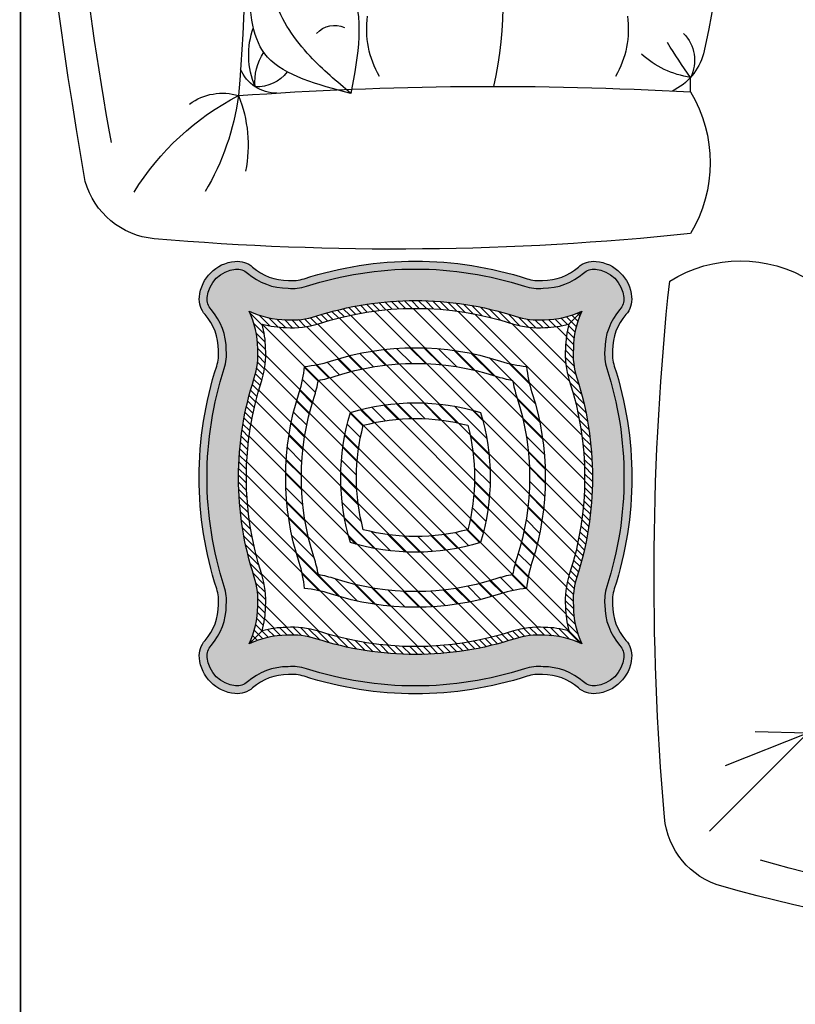
# Model space of a CAD drawing. Units: inches. Extents: x 844 to 2234, y 346 to 1084.
# Tile 50 of 93: x 1843 to 1859, y 668 to 688. Entities that reach past the tile are written whole.
import ezdxf

# ---------------------------------------------------------------- set-up
doc = ezdxf.new("R2010")
doc.units = ezdxf.units.IN
doc.header["$MEASUREMENT"] = 0
doc.layers.add('A-WALL', color=7, linetype='Continuous', lineweight=35)
doc.layers.add('furniture', color=8, linetype='Continuous', lineweight=18)
for name, color, linetype in [('RA-AP-01$0$FURN', 3, 'Continuous'), ('RA-AP-01$0$steel', 193, 'Continuous'), ('RA-AP-01$0$WOOD', 64, 'Continuous')]:
    doc.layers.add(name, color=color, linetype=linetype)
pattern_1 = [(45, (0, 1.362436106329781), (-0.0088388347648318, 0.0088388347648318), [])]
pattern_2 = [(45, (0, 1.362436106329781), (-0.0044194173824159, 0.0044194173824159), [])]

# ---------------------------------------------------------------- blocks, each defined once
blk = doc.blocks.new('A$C2FCF5309')
at = {"layer": 'RA-AP-01$0$FURN'}
h = blk.add_hatch(dxfattribs=at)
h.set_pattern_fill('ANSI31', color=256, scale=0.1, style=0)
h.set_pattern_definition(pattern_1)
h.paths.add_polyline_path([(5.038683893313746, -5.169250834004607, -0.1583983521602212), (5.038683893312098, -5.373464580902012, 0.0306258898943267), (5.033304057242972, -5.394827569605182, 0.0306258898948892), (5.01194106853941, -5.40020740567441, -0.1028142994996694), (4.878286182323899, -5.414871334512708), (4.863600873530158, -5.43331743520547, 0.1120482678681049), (5.018059823131753, -5.419248541734471, -0.052642197802937), (5.050972078299936, -5.412495590662115, -0.0526421977994963), (5.057725029371615, -5.379583335496025, 0.1583028414702701), (5.057725029372958, -5.163132079409654, -0.052642197806903), (5.050972078299777, -5.130219824239078, -0.0526421977995126), (5.018059823133679, -5.123466873167369, 0.0215995840215353), (4.988903013548211, -5.115372132362452), (4.975007495303644, -5.132826183367946, -0.0289147572844802), (5.011941068537408, -5.142508009226167, 0.0306258898976746), (5.033304057242868, -5.147887845296027, 0.0306258899022411)])
h.paths.add_polyline_path([(4.975007495303645, -5.132826183367946), (4.988903013548211, -5.115372132362452, 0.1362374241599938), (4.801608567045604, -5.12346687316654, -0.0526421978036853), (4.768696311876971, -5.130219824239102, -0.05264219780204), (4.761943360804856, -5.163132079406747, 0.1583028414743723), (4.761943360806116, -5.379583335498449, -0.0526421977955461), (4.768696311877141, -5.412495590662114, -0.0526421978073986), (4.801608567048022, -5.419248541735437, 0.0454484293938888), (4.863600873530158, -5.43331743520547), (4.878286182323899, -5.414871334512708, -0.0546933379798044), (4.80772732164382, -5.40020740567649, 0.030625889903973), (4.786364332934043, -5.394827569605216, 0.0306258898932853), (4.780984496865101, -5.373464580902791, -0.1583983521638281), (4.780984496864308, -5.169250834000963, 0.03062588989692), (4.786364332933943, -5.147887845296004, 0.0306258898946324), (4.807727321637318, -5.142508009226805, -0.1288932573266927)])
h.paths.add_polyline_path([(4.843422214712861, -5.204945727074827, -0.0783685831716868), (4.924134454130224, -5.196727409635105), (4.939146578618322, -5.177870798323143, 0.1012675676854134), (4.827248748758957, -5.188772261120899, 0.1253648873081696), (4.820394258584192, -5.327034652050361), (4.837127701354095, -5.306015906404253, -0.0981593964869636)], flags=17)
h.paths.add_polyline_path([(4.843422214712824, -5.337769687826355, -0.0311091841722656), (4.837127701354095, -5.306015906404253), (4.820394258584193, -5.32703465205036, 0.0247727657431944), (4.827248748758908, -5.353943153780261, 0.0812754385032542), (4.916962478476905, -5.36629034358622), (4.933684093813825, -5.345286454285511, -0.0876255421014372)], flags=17)
h.paths.add_polyline_path([(4.992419641418037, -5.353943153780226, 0.1506053783834298), (4.992419641417933, -5.188772261120954, 0.0485966419124224), (4.939146578618321, -5.177870798323143), (4.924134454130224, -5.196727409635105, -0.0507799419579301), (4.976246175464031, -5.204945727074882, -0.1296645318906876), (4.97624617546411, -5.337769687826316, -0.0415667119298777), (4.933684093813825, -5.345286454285511), (4.916962478476905, -5.36629034358622, 0.0684915676023693)], flags=17)
h = blk.add_hatch(dxfattribs=at)
h.set_pattern_fill('ANSI31', color=256, scale=0.1, style=0)
h.set_pattern_definition(pattern_1)
h.paths.add_polyline_path([(5.038683893313746, -5.169250834004607, -0.1583983521602212), (5.038683893312098, -5.373464580902012, 0.0306258898943267), (5.033304057242972, -5.394827569605182, 0.0306258898948892), (5.01194106853941, -5.40020740567441, -0.1028142994996694), (4.878286182323899, -5.414871334512708), (4.863600873530158, -5.43331743520547, 0.1120482678681049), (5.018059823131753, -5.419248541734471, -0.052642197802937), (5.050972078299936, -5.412495590662115, -0.0526421977994963), (5.057725029371615, -5.379583335496025, 0.1583028414702701), (5.057725029372958, -5.163132079409654, -0.052642197806903), (5.050972078299777, -5.130219824239078, -0.0526421977995126), (5.018059823133679, -5.123466873167369, 0.0215995840215353), (4.988903013548211, -5.115372132362452), (4.975007495303644, -5.132826183367946, -0.0289147572844802), (5.011941068537408, -5.142508009226167, 0.0306258898976746), (5.033304057242868, -5.147887845296027, 0.0306258899022411)])
h.paths.add_polyline_path([(4.975007495303645, -5.132826183367946), (4.988903013548211, -5.115372132362452, 0.1362374241599938), (4.801608567045604, -5.12346687316654, -0.0526421978036853), (4.768696311876971, -5.130219824239102, -0.05264219780204), (4.761943360804856, -5.163132079406747, 0.1583028414743723), (4.761943360806116, -5.379583335498449, -0.0526421977955461), (4.768696311877141, -5.412495590662114, -0.0526421978073986), (4.801608567048022, -5.419248541735437, 0.0454484293938888), (4.863600873530158, -5.43331743520547), (4.878286182323899, -5.414871334512708, -0.0546933379798044), (4.80772732164382, -5.40020740567649, 0.030625889903973), (4.786364332934043, -5.394827569605216, 0.0306258898932853), (4.780984496865101, -5.373464580902791, -0.1583983521638281), (4.780984496864308, -5.169250834000963, 0.03062588989692), (4.786364332933943, -5.147887845296004, 0.0306258898946324), (4.807727321637318, -5.142508009226805, -0.1288932573266927)])
h.paths.add_polyline_path([(4.843422214712861, -5.204945727074827, -0.0783685831716868), (4.924134454130224, -5.196727409635105), (4.939146578618322, -5.177870798323143, 0.1012675676854134), (4.827248748758957, -5.188772261120899, 0.1253648873081696), (4.820394258584192, -5.327034652050361), (4.837127701354095, -5.306015906404253, -0.0981593964869636)], flags=17)
h.paths.add_polyline_path([(4.843422214712824, -5.337769687826355, -0.0311091841722656), (4.837127701354095, -5.306015906404253), (4.820394258584193, -5.32703465205036, 0.0247727657431944), (4.827248748758908, -5.353943153780261, 0.0812754385032542), (4.916962478476905, -5.36629034358622), (4.933684093813825, -5.345286454285511, -0.0876255421014372)], flags=17)
h.paths.add_polyline_path([(4.992419641418037, -5.353943153780226, 0.1506053783834298), (4.992419641417933, -5.188772261120954, 0.0485966419124224), (4.939146578618321, -5.177870798323143), (4.924134454130224, -5.196727409635105, -0.0507799419579301), (4.976246175464031, -5.204945727074882, -0.1296645318906876), (4.97624617546411, -5.337769687826316, -0.0415667119298777), (4.933684093813825, -5.345286454285511), (4.916962478476905, -5.36629034358622, 0.0684915676023693)], flags=17)
at = {"layer": 'RA-AP-01$0$WOOD'}
h = blk.add_hatch(color=256, dxfattribs=at)
edge = h.paths.add_edge_path()
edge.add_arc((4.683001772622394, -5.026441828662609), 0.0299999999999998, 48.77105092035535, 95.25687599427813)
edge.add_arc((4.684834195088484, -5.046357707450686), 0.0499999999998897, 95.25687599443106, 174.7431240064049)
edge.add_arc((4.664918316300367, -5.044525284985046), 0.0300000000000005, 174.7431240062535, 221.2289490796905)
edge.add_arc((4.591236830209155, -5.109094338216345), 0.0679700159630267, -0.5333070513215148, 41.228949079691915, ccw=False)
edge.add_arc((4.609451302807284, -5.114694777173187), 0.0500000000000008, -17.3556839752095, 5.7020707654044145, ccw=False)
edge.add_arc((5.095208119646659, -5.271357707450659), 0.4603971832811796, 162.0683908477609, 197.9316091523306)
edge.add_arc((4.609451302807533, -5.428020637728902), 0.0500000000000006, -5.702070765320514, 17.355683975293914, ccw=False)
edge.add_arc((4.591236830209412, -5.433621076685779), 0.0679700159630261, -41.228949079600625, 0.5333070514128053, ccw=False)
edge.add_arc((4.664918316300727, -5.498190129916959), 0.0299999999999995, 138.7710509204022, 185.256875994324)
edge.add_arc((4.684834195088642, -5.496357707450695), 0.0499999999997451, 185.2568759946742, 264.74312400432)
edge.add_arc((4.683001772622394, -5.516273586238612), 0.03, 264.743124003969, 311.2289490796446)
edge.add_arc((4.747570825853633, -5.589955072329876), 0.0679700159630271, 89.4666929486321, 131.2289490796457, ccw=False)
edge.add_arc((4.753171264810493, -5.57174059973175), 0.0500000000000015, 72.64431602474701, 95.70207076536133, ccw=False)
edge.add_arc((4.909834195088355, -5.085983782892503), 0.4603971832811774, 252.0683908477147, 287.9316091522845)
edge.add_arc((5.06649712536621, -5.57174059973175), 0.0499999999999999, 84.29792923463953, 107.35568397525361, ccw=False)
edge.add_arc((5.072097564323069, -5.589955072329877), 0.0679700159630274, 48.771050920354185, 90.5333070513679, ccw=False)
edge.add_arc((5.136666617554309, -5.516273586238614), 0.0299999999999997, 228.771050920353, 275.2568759942969)
edge.add_arc((5.134834195088338, -5.496357707450417), 0.0499999999999982, 275.2568759942949, 354.7431240057633)
edge.add_arc((5.154750073876535, -5.498190129916372), 0.0299999999999999, 354.7431240057662, 401.2289490796891)
edge.add_arc((5.228431559967749, -5.433621076685074), 0.0679700159630274, 179.4666929486771, 221.2289490796903, ccw=False)
edge.add_arc((5.210217087369615, -5.428020637728227), 0.0499999999999976, 162.6443160247947, 185.7020707654089, ccw=False)
edge.add_arc((4.724460270530244, -5.271357707450757), 0.4603971832811793, 342.0683908477607, 377.9316091523305)
edge.add_arc((5.210217087369368, -5.114694777172509), 0.0500000000000019, 174.2979292346878, 197.355683975302, ccw=False)
edge.add_arc((5.228431559967489, -5.109094338215639), 0.0679700159630279, 138.7710509203993, 180.5333070514128, ccw=False)
edge.add_arc((5.154750073876174, -5.044525284984457), 0.0300000000000001, 318.771050920401, 365.2568759954636)
edge.add_arc((5.13483419508816, -5.046357707450624), 0.0499999999998349, 5.256875995237118, 84.74312400549572)
edge.add_arc((5.136666617554308, -5.026441828662608), 0.0299999999999994, 84.74312400572185, 131.2289490796446)
edge.add_arc((5.072097564323072, -4.952760342571343), 0.0679700159630261, 269.4666929486298, 311.22894907964354, ccw=False)
edge.add_arc((5.066497125366206, -4.97097481516947), 0.0499999999999992, 252.64431602475162, 275.70207076536565, ccw=False)
edge.add_arc((4.909834195088355, -5.456731632008717), 0.4603971832811764, 72.06839084771546, 107.9316091522853)
edge.add_arc((4.753171264810493, -4.970974815169471), 0.0500000000000016, 264.2979292346387, 287.355683975253, ccw=False)
edge.add_arc((4.747570825853633, -4.952760342571346), 0.0679700159630274, 228.7710509203543, 270.5333070513679, ccw=False)
edge = h.paths.add_edge_path(flags=16)
edge.add_arc((4.683001772622395, -5.026441828662608), 0.019999999999999, 48.7710509203555, 95.2568759942793)
edge.add_arc((4.684834195088469, -5.046357707450671), 0.0399999999998731, 95.2568759944489, 174.7431240064248)
edge.add_arc((4.664918316300404, -5.044525284985035), 0.020000000000036, 174.7431240062186, 221.2289490796461)
edge.add_arc((4.591236830209151, -5.109094338216346), 0.0779700159630296, -0.13764630038667747, 41.228949079689585, ccw=False)
edge.add_arc((4.609451302807307, -5.11469477717304), 0.060000000000024, -17.406127045137907, 5.176192161068002, ccw=False)
edge.add_arc((5.09520811964665, -5.271357707450659), 0.4503971832811708, 162.0623235129628, 197.9376764869162)
edge.add_arc((4.609451302807532, -5.428020637728943), 0.0599999999999982, -5.176192160466428, 17.406127046715312, ccw=False)
edge.add_arc((4.591236830209414, -5.433621076685778), 0.0779700159630257, -41.2289490796029, 0.13764630095249686, ccw=False)
edge.add_arc((4.664918316300731, -5.498190129916961), 0.0200000000000047, 138.7710509204103, 185.2568759943212)
edge.add_arc((4.684834195088606, -5.496357707450731), 0.0399999999997066, 185.2568759947174, 264.7431240043665)
edge.add_arc((4.683001772622369, -5.516273586238541), 0.020000000000069, 264.7431240038842, 311.2289490795622)
edge.add_arc((4.747570825853635, -5.589955072329884), 0.0779700159630344, 89.8623536987642, 131.2289490796432, ccw=False)
edge.add_arc((4.753171264810603, -5.571740599731771), 0.0599999999999895, 72.5938729544394, 95.1761921602253, ccw=False)
edge.add_arc((4.909834195088365, -5.085983782892505), 0.4503971832811724, 252.0623235129989, 287.9376764870498)
edge.add_arc((5.066497125366216, -5.571740599731755), 0.0600000000000047, 84.8238078399923, 107.40612704528041, ccw=False)
edge.add_arc((5.072097564322998, -5.589955072329853), 0.077970015963056, 48.771050920303594, 90.13764630126451, ccw=False)
edge.add_arc((5.136666617554307, -5.516273586238622), 0.0199999999999931, 228.771050920344, 275.2568759943037)
edge.add_arc((5.134834195088338, -5.496357707450416), 0.0400000000000004, 275.2568759942928, 354.7431240057607)
edge.add_arc((5.154750073876533, -5.498190129916375), 0.0200000000000037, 354.7431240057783, 401.2289490796939)
edge.add_arc((5.228431559967745, -5.433621076685076), 0.0779700159630239, 179.8623536995147, 221.2289490796908, ccw=False)
edge.add_arc((5.210217087369586, -5.428020637728345), 0.0600000000000054, 162.5938729554486, 185.1761921609759, ccw=False)
edge.add_arc((4.724460270530243, -5.271357707450766), 0.4503971832811826, 342.0623235128896, 377.937676486982)
edge.add_arc((5.210217087369347, -5.114694777172486), 0.0599999999999777, 174.8238078387611, 197.4061270462219, ccw=False)
edge.add_arc((5.228431559967523, -5.109094338215542), 0.0779700159629885, 138.7710509204687, 180.1376463004423, ccw=False)
edge.add_arc((5.154750073876175, -5.044525284984459), 0.0199999999999989, 318.771050920406, 365.2568759954698)
edge.add_arc((5.134834195088138, -5.046357707450646), 0.0399999999998586, 5.256875995208452, 84.74312400546732)
edge.add_arc((5.136666617554292, -5.02644182866256), 0.0199999999999529, 84.74312400577769, 131.2289490797025)
edge.add_arc((5.072097564323069, -4.952760342571338), 0.077970015963032, 269.86235369901414, 311.2289490796421, ccw=False)
edge.add_arc((5.06649712536618, -4.97097481516946), 0.0600000000000007, 252.5938729548277, 275.17619216047467, ccw=False)
edge.add_arc((4.909834195088353, -5.456731632008716), 0.4503971832811739, 72.06232351293887, 107.9376764867365)
edge.add_arc((4.753171264810429, -4.970974815169467), 0.0599999999999991, 264.82380783985815, 287.40612704769893, ccw=False)
edge.add_arc((4.747570825853681, -4.952760342571361), 0.0779700159630467, 228.7710509203206, 270.13764630113724, ccw=False)
h = blk.add_hatch(color=256, dxfattribs=at)
edge = h.paths.add_edge_path()
edge.add_arc((4.683001772622395, -5.026441828662608), 0.019999999999999, 48.7710509203555, 95.2568759942793)
edge.add_arc((4.684834195088469, -5.046357707450671), 0.0399999999998731, 95.2568759944489, 174.7431240064248)
edge.add_arc((4.664918316300404, -5.044525284985035), 0.020000000000036, 174.7431240062186, 221.2289490796461)
edge.add_arc((4.591236830209151, -5.109094338216346), 0.0779700159630296, -0.13764630038667747, 41.228949079689585, ccw=False)
edge.add_arc((4.609451302807307, -5.11469477717304), 0.060000000000024, -17.406127045137907, 5.176192161068002, ccw=False)
edge.add_arc((5.09520811964665, -5.271357707450659), 0.4503971832811708, 162.0623235129628, 197.9376764869162)
edge.add_arc((4.609451302807532, -5.428020637728943), 0.0599999999999982, -5.176192160466428, 17.406127046715312, ccw=False)
edge.add_arc((4.591236830209414, -5.433621076685778), 0.0779700159630257, -41.2289490796029, 0.13764630095249686, ccw=False)
edge.add_arc((4.664918316300731, -5.498190129916961), 0.0200000000000047, 138.7710509204103, 185.2568759943212)
edge.add_arc((4.684834195088606, -5.496357707450731), 0.0399999999997066, 185.2568759947174, 264.7431240043665)
edge.add_arc((4.683001772622369, -5.516273586238541), 0.020000000000069, 264.7431240038842, 311.2289490795622)
edge.add_arc((4.747570825853635, -5.589955072329884), 0.0779700159630344, 89.8623536987642, 131.2289490796432, ccw=False)
edge.add_arc((4.753171264810603, -5.571740599731771), 0.0599999999999895, 72.5938729544394, 95.1761921602253, ccw=False)
edge.add_arc((4.909834195088365, -5.085983782892505), 0.4503971832811724, 252.0623235129989, 287.9376764870498)
edge.add_arc((5.066497125366216, -5.571740599731755), 0.0600000000000047, 84.8238078399923, 107.40612704528041, ccw=False)
edge.add_arc((5.072097564322998, -5.589955072329853), 0.077970015963056, 48.771050920303594, 90.13764630126451, ccw=False)
edge.add_arc((5.136666617554307, -5.516273586238622), 0.0199999999999931, 228.771050920344, 275.2568759943037)
edge.add_arc((5.134834195088338, -5.496357707450416), 0.0400000000000004, 275.2568759942928, 354.7431240057607)
edge.add_arc((5.154750073876533, -5.498190129916375), 0.0200000000000037, 354.7431240057783, 401.2289490796939)
edge.add_arc((5.228431559967745, -5.433621076685076), 0.0779700159630239, 179.8623536995147, 221.2289490796908, ccw=False)
edge.add_arc((5.210217087369586, -5.428020637728345), 0.0600000000000054, 162.5938729554486, 185.1761921609759, ccw=False)
edge.add_arc((4.724460270530243, -5.271357707450766), 0.4503971832811826, 342.0623235128896, 377.937676486982)
edge.add_arc((5.210217087369347, -5.114694777172486), 0.0599999999999777, 174.8238078387611, 197.4061270462219, ccw=False)
edge.add_arc((5.228431559967523, -5.109094338215542), 0.0779700159629885, 138.7710509204687, 180.1376463004423, ccw=False)
edge.add_arc((5.154750073876175, -5.044525284984459), 0.0199999999999989, 318.771050920406, 365.2568759954698)
edge.add_arc((5.134834195088138, -5.046357707450646), 0.0399999999998586, 5.256875995208452, 84.74312400546732)
edge.add_arc((5.136666617554292, -5.02644182866256), 0.0199999999999529, 84.74312400577769, 131.2289490797025)
edge.add_arc((5.072097564323069, -4.952760342571338), 0.077970015963032, 269.86235369901414, 311.2289490796421, ccw=False)
edge.add_arc((5.06649712536618, -4.97097481516946), 0.0600000000000007, 252.5938729548277, 275.17619216047467, ccw=False)
edge.add_arc((4.909834195088353, -5.456731632008716), 0.4503971832811739, 72.06232351293887, 107.9376764867365)
edge.add_arc((4.753171264810429, -4.970974815169467), 0.0599999999999991, 264.82380783985815, 287.40612704769893, ccw=False)
edge.add_arc((4.747570825853681, -4.952760342571361), 0.0779700159630467, 228.7710509203206, 270.13764630113724, ccw=False)
edge = h.paths.add_edge_path(flags=16)
edge.add_arc((4.591236830209151, -5.109094338216348), 0.1179700159630308, 0.7417751874182841, 24.563326950263672, ccw=False)
edge.add_arc((4.609451302807302, -5.114694777173093), 0.100000000000012, -17.52836504564658, 4.087328884225087, ccw=False)
edge.add_arc((5.095208119646651, -5.271357707450657), 0.4103971832811724, 162.0403002448777, 197.9596997550675)
edge.add_arc((4.60945130280753, -5.428020637728918), 0.1000000000000027, -4.087328883827581, 17.528365046291924, ccw=False)
edge.add_arc((4.591236830209414, -5.433621076685779), 0.1179700159630246, 335.43667305041845, 359.2582248129738, ccw=False)
edge.add_arc((4.747570825853596, -5.589955072329891), 0.117970015963042, 90.7417751868461, 114.5633269496104, ccw=False)
edge.add_arc((4.753171264810559, -5.571740599731767), 0.0999999999999976, 72.47163495370341, 94.0873288836737, ccw=False)
edge.add_arc((4.909834195088367, -5.085983782892503), 0.4103971832811735, 252.0403002449999, 287.9596997551833)
edge.add_arc((5.066497125366205, -5.571740599731755), 0.1000000000000057, 85.91267111645209, 107.5283650455624, ccw=False)
edge.add_arc((5.072097564322985, -5.58995507232986), 0.117970015963046, 65.4366730497672, 89.25822481317113, ccw=False)
edge.add_arc((5.22843155996773, -5.433621076684992), 0.1179700159630096, 180.7417751873964, 204.5633269502712, ccw=False)
edge.add_arc((5.210217087369591, -5.428020637728301), 0.0999999999999969, 162.4716349546276, 184.0873288841682, ccw=False)
edge.add_arc((4.724460270530243, -5.271357707450766), 0.4103971832811825, 342.0403002448147, 377.9596997550345)
edge.add_arc((5.210217087369347, -5.114694777172489), 0.0999999999999796, 175.9126711156995, 197.5283650464392, ccw=False)
edge.add_arc((5.228431559967512, -5.109094338215525), 0.1179700159630019, 155.4366730502992, 179.2582248126247, ccw=False)
edge.add_arc((5.072097564323172, -4.952760342571314), 0.1179700159630537, 270.74177518697286, 294.56332694975765, ccw=False)
edge.add_arc((5.066497125366189, -4.970974815169462), 0.1000000000000017, 252.471634954247, 274.0873288838353, ccw=False)
edge.add_arc((4.909834195088353, -5.456731632008716), 0.4103971832811758, 72.04030024486342, 107.9596997549354)
edge.add_arc((4.75317126481046, -4.970974815169467), 0.1000000000000041, 265.91267111635307, 287.5283650466103, ccw=False)
edge.add_arc((4.747570825853629, -4.952760342571342), 0.1179700159630538, 245.43667304992562, 269.2582248131125, ccw=False)
h = blk.add_hatch(dxfattribs=at)
h.set_pattern_fill('ANSI31', color=256, scale=0.05, style=0)
h.set_pattern_definition(pattern_2)
h.paths.add_polyline_path([(5.105336294329346, -5.394854099602528, 0.0940138826956367), (5.100476366643778, -5.435568764288975, 0.0606271852326483), (5.104678567100611, -5.466202079462671, 0.0606271852344644), (5.074045251925975, -5.46199987900586, 0.0940138827021426), (5.033330587236848, -5.466859806692645, -0.1305325492494615), (4.828072633169377, -5.477944178050054), (4.821119726105699, -5.486677669841435, 0.1336226599878005), (5.036379334063467, -5.476383803188216, -0.0945969211935747), (5.073624810952389, -5.471994942692536, -0.1043170707892296), (5.121137550891356, -5.48266106325342, -0.1043170707868944), (5.110471430330457, -5.435148323315565, -0.0945969211952573), (5.114860290825935, -5.397902846425963, 0.1580239521433527), (5.114860290826324, -5.144812568476775, -0.0945969212010491), (5.110471430330247, -5.10756709158498, -0.1043170707844371), (5.121137550890657, -5.060054351648168, -0.104317070786514), (5.073624810952866, -5.070720472208642, -0.0945969211958523), (5.036379334063063, -5.066331611712874, 0.1580239521426795), (4.783289056114906, -5.066331611712465, -0.0945969211985319), (4.746043579224103, -5.070720472208672, -0.1043170707882665), (4.698530839285552, -5.060054351647925, -0.1043170707867205), (4.709196959846443, -5.10756709158571, -0.094596921196788), (4.704808099350826, -5.144812568475902, 0.1580239521433127), (4.704808099350699, -5.397902846425022, -0.094596921197841), (4.709196959846712, -5.435148323315576, -0.1043170707855109), (4.698530839286393, -5.482661063252921, -0.1043170707864168), (4.746043579224162, -5.471994942692571, -0.0945969211977586), (4.783289056114671, -5.476383803188671, 0.0238966994662183), (4.821119726105699, -5.486677669841435), (4.828072633169378, -5.477944178050054, -0.0269814195959459), (4.786337802940177, -5.466859806692736, 0.0940138827039629), (4.745623138250268, -5.461999879005895, 0.0606271852320776), (4.714989823076826, -5.466202079462476, 0.0606271852304618), (4.719192023533341, -5.435568764289856, 0.0940138826917763), (4.714332095848404, -5.394854099604977, -0.1580706864542086), (4.714332095846561, -5.147861315302034, 0.0940138827032017), (4.719192023533127, -5.107146650612438, 0.0606271852329446), (4.714989823076289, -5.076513335438588, 0.0606271852340035), (4.745623138250698, -5.08071553589536, 0.0940138827025969), (4.786337802940015, -5.075855608208526, -0.1580706864508517), (5.033330587237968, -5.075855608208939, 0.0940138827009578), (5.074045251926627, -5.080715535895319, 0.0606271852322557), (5.104678567100159, -5.076513335438697, 0.0606271852308743), (5.100476366643561, -5.107146650611519, 0.0940138827178109), (5.105336294331983, -5.147861315307182, -0.1580706864490946)])
h = blk.add_hatch(dxfattribs=at)
h.set_pattern_fill('ANSI31', color=256, scale=0.05, style=0)
h.set_pattern_definition(pattern_2)
h.paths.add_polyline_path([(5.105336294329346, -5.394854099602528, 0.0940138826956367), (5.100476366643778, -5.435568764288975, 0.0606271852326483), (5.104678567100611, -5.466202079462671, 0.0606271852344644), (5.074045251925975, -5.46199987900586, 0.0940138827021426), (5.033330587236848, -5.466859806692645, -0.1305325492494615), (4.828072633169377, -5.477944178050054), (4.821119726105699, -5.486677669841435, 0.1336226599878005), (5.036379334063467, -5.476383803188216, -0.0945969211935747), (5.073624810952389, -5.471994942692536, -0.1043170707892296), (5.121137550891356, -5.48266106325342, -0.1043170707868944), (5.110471430330457, -5.435148323315565, -0.0945969211952573), (5.114860290825935, -5.397902846425963, 0.1580239521433527), (5.114860290826324, -5.144812568476775, -0.0945969212010491), (5.110471430330247, -5.10756709158498, -0.1043170707844371), (5.121137550890657, -5.060054351648168, -0.104317070786514), (5.073624810952866, -5.070720472208642, -0.0945969211958523), (5.036379334063063, -5.066331611712874, 0.1580239521426795), (4.783289056114906, -5.066331611712465, -0.0945969211985319), (4.746043579224103, -5.070720472208672, -0.1043170707882665), (4.698530839285552, -5.060054351647925, -0.1043170707867205), (4.709196959846443, -5.10756709158571, -0.094596921196788), (4.704808099350826, -5.144812568475902, 0.1580239521433127), (4.704808099350699, -5.397902846425022, -0.094596921197841), (4.709196959846712, -5.435148323315576, -0.1043170707855109), (4.698530839286393, -5.482661063252921, -0.1043170707864168), (4.746043579224162, -5.471994942692571, -0.0945969211977586), (4.783289056114671, -5.476383803188671, 0.0238966994662183), (4.821119726105699, -5.486677669841435), (4.828072633169378, -5.477944178050054, -0.0269814195959459), (4.786337802940177, -5.466859806692736, 0.0940138827039629), (4.745623138250268, -5.461999879005895, 0.0606271852320776), (4.714989823076826, -5.466202079462476, 0.0606271852304618), (4.719192023533341, -5.435568764289856, 0.0940138826917763), (4.714332095848404, -5.394854099604977, -0.1580706864542086), (4.714332095846561, -5.147861315302034, 0.0940138827032017), (4.719192023533127, -5.107146650612438, 0.0606271852329446), (4.714989823076289, -5.076513335438588, 0.0606271852340035), (4.745623138250698, -5.08071553589536, 0.0940138827025969), (4.786337802940015, -5.075855608208526, -0.1580706864508517), (5.033330587237968, -5.075855608208939, 0.0940138827009578), (5.074045251926627, -5.080715535895319, 0.0606271852322557), (5.104678567100159, -5.076513335438697, 0.0606271852308743), (5.100476366643561, -5.107146650611519, 0.0940138827178109), (5.105336294331983, -5.147861315307182, -0.1580706864490946)])
h = blk.add_hatch(dxfattribs=at)
h.set_pattern_fill('ANSI32,_I', color=256, scale=0.1, style=2)
h.set_pattern_definition([(45, (0, 0), (-0.0265165042944955, 0.0265165042944955), []), (45, (0.0176776695, 0), (-0.0265165042944955, 0.0265165042944955), [])])
h.paths.add_polyline_path([(4.843422214712824, -5.337769687826354, 0.1296645318905289), (4.97624617546411, -5.337769687826316, 0.1296645318906876), (4.976246175464032, -5.204945727074882, 0.129664531890418), (4.843422214712861, -5.204945727074827, 0.129664531890765)], flags=0)
h.paths.add_polyline_path([(5.039131224122924, -5.170637849998464, -0.0326520429852175), (5.033304057242868, -5.147887845296027, -0.0326520429894721), (5.010554052537512, -5.142060678415043, 0.1561383235202698), (4.809114337641437, -5.142060678414318, -0.0326520429925972), (4.786364332933944, -5.147887845296004, -0.0326520429914489), (4.780537166052582, -5.170637850002729, 0.1561383235189577), (4.780537166052134, -5.37207756489719, -0.0326520429934175), (4.786364332934042, -5.394827569605215, -0.0326520429823496), (4.809114337634529, -5.400654736484653, 0.156138323524066), (5.010554052535268, -5.400654736486903, -0.032652042992888), (5.033304057242972, -5.394827569605183, -0.0326520429928733), (5.039131224124712, -5.372077564897496, 0.1561383235226786)], flags=0)
h.paths.add_polyline_path([(4.992419641418037, -5.353943153780226, -0.1506053783832862), (4.827248748758909, -5.353943153780261, -0.1506053783835069), (4.827248748758957, -5.188772261120899, -0.1506053783831346), (4.992419641417933, -5.188772261120954, -0.1506053783834298)], flags=0)
h.paths.add_polyline_path([(4.976246175464111, -5.337769687826316, -0.1296645318905298), (4.843422214712824, -5.337769687826354, -0.129664531890765), (4.843422214712862, -5.204945727074827, -0.1296645318904162), (4.976246175464031, -5.204945727074882, -0.1296645318906876)], flags=0)
h.paths.add_polyline_path([(5.105721254232479, -5.149054940982025, -0.0968902512052664), (5.100476366643561, -5.107146650611519, -0.0606271852308743), (5.104678567100159, -5.076513335438697, -0.0606271852322574), (5.074045251926626, -5.080715535895319, -0.0968902512197216), (5.032136961550132, -5.075470648304253, 0.1564657949319774), (4.787531428625239, -5.075470648304682, -0.0968902512150626), (4.745623138250699, -5.08071553589536, -0.060627185234009), (4.714989823076288, -5.076513335438587, -0.0606271852329501), (4.719192023533127, -5.10714665061244, -0.0968902512185585), (4.713947135942331, -5.149054940988458, 0.1564657949285579), (4.713947135940853, -5.393660473908259, -0.0968902512319826), (4.71919202353334, -5.435568764289873, -0.0606271852304288), (4.714989823076825, -5.466202079462476, -0.0606271852320811), (4.745623138250269, -5.461999879005895, -0.0968902512162649), (4.787531428625332, -5.467244766596559, 0.1564657949327057), (5.032136961551311, -5.46724476659659, -0.0968902512153659), (5.074045251925975, -5.46199987900586, -0.0606271852344627), (5.10467856710061, -5.466202079462671, -0.0606271852326483), (5.100476366643777, -5.435568764288975, -0.0968902512258216), (5.105721254235559, -5.393660473909953, 0.1564657949340142)])
h.paths.add_polyline_path([(5.057725029371625, -5.379583335495999, 0.0526421977995391), (5.050972078299936, -5.412495590662114, 0.0526421978029782), (5.018059823131728, -5.419248541734479, -0.1583028414681072), (4.801608567048168, -5.419248541735485, 0.0526421978076402), (4.76869631187714, -5.412495590662113, 0.0526421977956189), (4.761943360806101, -5.379583335498404, -0.1583028414743129), (4.761943360804846, -5.163132079406778, 0.0526421978020944), (4.768696311876972, -5.130219824239101, 0.0526421978033651), (4.80160856704541, -5.123466873166602, -0.1583028414716875), (5.018059823133628, -5.123466873167353, 0.0526421977995944), (5.050972078299776, -5.130219824239078, 0.0526421978070423), (5.057725029372986, -5.163132079409739, -0.1583028414701848)], flags=16)
h.paths.add_polyline_path([(5.038683893312112, -5.373464580901968, 0.0306258898943915), (5.033304057242972, -5.394827569605182, 0.0306258898948892), (5.01194106853941, -5.40020740567441, -0.1583983521587032), (4.807727321643864, -5.400207405676503, 0.0306258899040366), (4.786364332934043, -5.394827569605215, 0.0306258898931986), (4.780984496865119, -5.37346458090285, -0.1583983521638542), (4.7809844968643, -5.169250834000989, 0.0306258898969596), (4.786364332933945, -5.147887845296004, 0.0306258898946195), (4.807727321637311, -5.142508009226808, -0.1583983521623412), (5.011941068537318, -5.142508009226139, 0.030625889897807), (5.033304057242868, -5.147887845296028, 0.0306258899020632), (5.038683893313706, -5.169250834004486, -0.1583983521602835)], flags=0)
for p, q in [((4.714989823076289, -5.076513335438588), (4.698530839285552, -5.060054351647925)), ((4.714989823076289, -5.076513335438588), (4.698530839285552, -5.060054351647925)), ((5.104678567100159, -5.076513335438697), (5.121137550890656, -5.060054351648169)), ((5.104678567100159, -5.076513335438697), (5.121137550890656, -5.060054351648169)), ((5.10467856710061, -5.466202079462671), (5.121137550891355, -5.482661063253419)), ((5.10467856710061, -5.466202079462671), (5.121137550891355, -5.482661063253419))]:
    blk.add_line(p, q, dxfattribs=at)
for points in [[(4.702773858784635, -5.003879368495489, 0.2056608120285223), (4.680253138923443, -4.996568010480312, 0.3614336704708569), (4.635044498118043, -5.041776651286372, 0.2056608120263112), (4.642355856133262, -5.064297371147306, -0.1842662638101064), (4.65920390179375, -5.10972699154053, -0.1009492694051416), (4.657174869772992, -5.129609908955028, 0.1577727036674954), (4.657174869773219, -5.41310550594699, -0.1009492694051416), (4.659203901794006, -5.432988423361486, -0.1842662638101064), (4.64235585613359, -5.478418043754737, 0.2056608120285221), (4.635044498118431, -5.500938763615934, 0.3614336704593693), (4.680253138922529, -5.546147404420826, 0.2056608120364936), (4.702773858784635, -5.538836046405732, -0.1842662638101064), (4.748203479177874, -5.52198800074528, -0.1009492694051415), (4.768086396592371, -5.524017032766053, 0.1577727036674954), (5.051581993584332, -5.524017032766055, -0.1009492694051416), (5.071464910998829, -5.521988000745282, -0.1842662638101064), (5.116894531392067, -5.538836046405734, 0.2056608120286145), (5.13941525125327, -5.546147404420911, 0.3614336704683636), (5.184623892058835, -5.500938763615299, 0.2056608120285223), (5.177312534043641, -5.478418043754112, -0.1842662638101063), (5.160464488383153, -5.432988423360887, -0.1009492694051416), (5.162493520403909, -5.41310550594639, 0.1577727036674954), (5.162493520403684, -5.129609908954428, -0.1009492694051416), (5.160464488382894, -5.109726991539933, -0.1842662638101064), (5.17731253404331, -5.064297371146681, 0.2056608120337072), (5.184623892058415, -5.041776651284888, 0.3614336704623863), (5.139415251253259, -4.99656801048031, 0.2056608120285223), (5.116894531392067, -5.003879368495487, -0.1842662638101064), (5.071464910998829, -5.020727414155937, -0.1009492694051416), (5.051581993584332, -5.018698382135166, 0.1577727036674956), (4.768086396592371, -5.018698382135168, -0.1009492694051416), (4.748203479177874, -5.020727414155941, -0.1842662638101064)], [(4.702773858784635, -5.003879368495489, 0.2056608120285223), (4.680253138923443, -4.996568010480312, 0.3614336704708569), (4.635044498118043, -5.041776651286372, 0.2056608120263112), (4.642355856133262, -5.064297371147306, -0.1842662638101064), (4.65920390179375, -5.10972699154053, -0.1009492694051416), (4.657174869772992, -5.129609908955028, 0.1577727036674954), (4.657174869773219, -5.41310550594699, -0.1009492694051416), (4.659203901794006, -5.432988423361486, -0.1842662638101064), (4.64235585613359, -5.478418043754737, 0.2056608120285221), (4.635044498118431, -5.500938763615934, 0.3614336704593693), (4.680253138922529, -5.546147404420826, 0.2056608120364936), (4.702773858784635, -5.538836046405732, -0.1842662638101064), (4.748203479177874, -5.52198800074528, -0.1009492694051415), (4.768086396592371, -5.524017032766053, 0.1577727036674954), (5.051581993584332, -5.524017032766055, -0.1009492694051416), (5.071464910998829, -5.521988000745282, -0.1842662638101064), (5.116894531392067, -5.538836046405734, 0.2056608120286145), (5.13941525125327, -5.546147404420911, 0.3614336704683636), (5.184623892058835, -5.500938763615299, 0.2056608120285223), (5.177312534043641, -5.478418043754112, -0.1842662638101063), (5.160464488383153, -5.432988423360887, -0.1009492694051416), (5.162493520403909, -5.41310550594639, 0.1577727036674954), (5.162493520403684, -5.129609908954428, -0.1009492694051416), (5.160464488382894, -5.109726991539933, -0.1842662638101064), (5.17731253404331, -5.064297371146681, 0.2056608120337072), (5.184623892058415, -5.041776651284888, 0.3614336704623863), (5.139415251253259, -4.99656801048031, 0.2056608120285223), (5.116894531392067, -5.003879368495487, -0.1842662638101064), (5.071464910998829, -5.020727414155937, -0.1009492694051416), (5.051581993584332, -5.018698382135166, 0.1577727036674956), (4.768086396592371, -5.018698382135168, -0.1009492694051416), (4.748203479177874, -5.020727414155941, -0.1842662638101064)], [(4.696183163397222, -5.011400188551196, 0.2056608120285295), (4.681169350156427, -5.006525949874411, 0.3614336704708588), (4.645002437512154, -5.042692862519237, 0.2056608120262659), (4.649876676188964, -5.057706675759887, -0.182481815856965), (4.669206621172843, -5.109281651732388, -0.0988540857970112), (4.666703803477437, -5.13264334722805, 0.1578269695851905), (4.666703803477144, -5.410072067672365, -0.0988540858013112), (4.6692066211731, -5.433433763168966, -0.1824818158591246), (4.649876676189301, -5.485008739142145, 0.2056608120284717), (4.64500243751253, -5.500022552382944, 0.3614336704593821), (4.681169350155757, -5.536189465026749, 0.2056608120365057), (4.696183163397221, -5.531315226350026, -0.1824818158605826), (4.747758139370833, -5.51198528136619, -0.0988540857951607), (4.771119834866025, -5.514488099061806, 0.1578269695856264), (5.04854855531107, -5.514488099061688, -0.0988540857929677), (5.071910250805761, -5.511985281366138, -0.1824818158609529), (5.123485226779481, -5.531315226350027, 0.2056608120286893), (5.138499040020282, -5.536189465026812, 0.3614336704683556), (5.174665952664737, -5.500022552382323, 0.2056608120284882), (5.169791713987938, -5.485008739141532, -0.1824818158574124), (5.150461769004059, -5.4334337631689, -0.0988540857940221), (5.152964586699289, -5.410072067673927, 0.1578269695858123), (5.1529645866996, -5.132643347228565, -0.0988540858025403), (5.150461769003872, -5.109281651731659, -0.1824818158565006), (5.169791713987599, -5.057706675759273, 0.2056608120337192), (5.174665952664335, -5.042692862518078, 0.3614336704623903), (5.138499040020236, -5.006525949874406, 0.2056608120285323), (5.123485226779481, -5.011400188551195, -0.1824818158594503), (5.071910250806212, -5.03073013353503, -0.09885408579455), (5.048548555311143, -5.028227315839558, 0.1578269695844942), (4.771119834867991, -5.028227315838772, -0.0988540858042156), (4.747758139370745, -5.030730133535067, -0.1824818158603032)], [(4.696183163397222, -5.011400188551196, 0.2056608120285295), (4.681169350156427, -5.006525949874411, 0.3614336704708588), (4.645002437512154, -5.042692862519237, 0.2056608120262659), (4.649876676188964, -5.057706675759887, -0.182481815856965), (4.669206621172843, -5.109281651732388, -0.0988540857970112), (4.666703803477437, -5.13264334722805, 0.1578269695851905), (4.666703803477144, -5.410072067672365, -0.0988540858013112), (4.6692066211731, -5.433433763168966, -0.1824818158591246), (4.649876676189301, -5.485008739142145, 0.2056608120284717), (4.64500243751253, -5.500022552382944, 0.3614336704593821), (4.681169350155757, -5.536189465026749, 0.2056608120365057), (4.696183163397221, -5.531315226350026, -0.1824818158605826), (4.747758139370833, -5.51198528136619, -0.0988540857951607), (4.771119834866025, -5.514488099061806, 0.1578269695856264), (5.04854855531107, -5.514488099061688, -0.0988540857929677), (5.071910250805761, -5.511985281366138, -0.1824818158609529), (5.123485226779481, -5.531315226350027, 0.2056608120286893), (5.138499040020282, -5.536189465026812, 0.3614336704683556), (5.174665952664737, -5.500022552382323, 0.2056608120284882), (5.169791713987938, -5.485008739141532, -0.1824818158574124), (5.150461769004059, -5.4334337631689, -0.0988540857940221), (5.152964586699289, -5.410072067673927, 0.1578269695858123), (5.1529645866996, -5.132643347228565, -0.0988540858025403), (5.150461769003872, -5.109281651731659, -0.1824818158565006), (5.169791713987599, -5.057706675759273, 0.2056608120337192), (5.174665952664335, -5.042692862518078, 0.3614336704623903), (5.138499040020236, -5.006525949874406, 0.2056608120285323), (5.123485226779481, -5.011400188551195, -0.1824818158594503), (5.071910250806212, -5.03073013353503, -0.09885408579455), (5.048548555311143, -5.028227315839558, 0.1578269695844942), (4.771119834867991, -5.028227315838772, -0.0988540858042156), (4.747758139370745, -5.030730133535067, -0.1824818158603032)], [(4.698530839285552, -5.060054351647925, -0.1043170707867612), (4.709196959846444, -5.107567091585729, -0.0945969211969405), (4.704808099350802, -5.144812568475978, 0.1580239521432241), (4.704808099350681, -5.397902846424963, -0.0945969211980322), (4.709196959846711, -5.43514832331559, -0.104317070785482), (4.698530839286393, -5.482661063252921, -0.1043170707864036), (4.746043579224155, -5.471994942692571, -0.094596921197375), (4.78328905611452, -5.476383803188623, 0.1580239521431959), (5.036379334063463, -5.476383803188218, -0.0945969211935888), (5.07362481095239, -5.471994942692536, -0.1043170707892253), (5.121137550891355, -5.482661063253419, -0.1043170707868921), (5.110471430330457, -5.435148323315565, -0.0945969211954828), (5.114860290825962, -5.397902846425878, 0.158023952143358), (5.114860290826295, -5.144812568476682, -0.0945969212007617), (5.110471430330247, -5.107567091584995, -0.1043170707844689), (5.121137550890656, -5.060054351648169, -0.1043170707864946), (5.073624810952874, -5.070720472208642, -0.0945969211956941), (5.036379334063131, -5.066331611712896, 0.1580239521426976), (4.783289056114946, -5.066331611712452, -0.0945969211986379), (4.746043579224103, -5.070720472208672, -0.1043170707882684)], [(4.698530839285552, -5.060054351647925, -0.1043170707867612), (4.709196959846444, -5.107567091585729, -0.0945969211969405), (4.704808099350802, -5.144812568475978, 0.1580239521432241), (4.704808099350681, -5.397902846424963, -0.0945969211980322), (4.709196959846711, -5.43514832331559, -0.104317070785482), (4.698530839286393, -5.482661063252921, -0.1043170707864036), (4.746043579224155, -5.471994942692571, -0.094596921197375), (4.78328905611452, -5.476383803188623, 0.1580239521431959), (5.036379334063463, -5.476383803188218, -0.0945969211935888), (5.07362481095239, -5.471994942692536, -0.1043170707892253), (5.121137550891355, -5.482661063253419, -0.1043170707868921), (5.110471430330457, -5.435148323315565, -0.0945969211954828), (5.114860290825962, -5.397902846425878, 0.158023952143358), (5.114860290826295, -5.144812568476682, -0.0945969212007617), (5.110471430330247, -5.107567091584995, -0.1043170707844689), (5.121137550890656, -5.060054351648169, -0.1043170707864946), (5.073624810952874, -5.070720472208642, -0.0945969211956941), (5.036379334063131, -5.066331611712896, 0.1580239521426976), (4.783289056114946, -5.066331611712452, -0.0945969211986379), (4.746043579224103, -5.070720472208672, -0.1043170707882684)], [(4.714989823076289, -5.076513335438588, -0.0606271852329464), (4.719192023533127, -5.107146650612439, -0.0940138827030756), (4.714332095846578, -5.147861315301983, 0.1580706864542707), (4.714332095848417, -5.394854099605018, -0.0940138826916965), (4.719192023533341, -5.435568764289864, -0.0606271852304462), (4.714989823076826, -5.466202079462476, -0.0606271852320585), (4.745623138250258, -5.461999879005895, -0.0940138827037036), (4.786337802940059, -5.466859806692699, 0.1580706864500221), (5.033330587236783, -5.466859806692666, -0.0940138827023111), (5.074045251925979, -5.46199987900586, -0.060627185234454), (5.10467856710061, -5.466202079462671, -0.0606271852326709), (5.100476366643777, -5.435568764288963, -0.0940138826958686), (5.105336294329379, -5.394854099602421, 0.1580706864489859), (5.105336294331999, -5.147861315307237, -0.0940138827179432), (5.100476366643561, -5.107146650611518, -0.0606271852308726), (5.104678567100159, -5.076513335438697, -0.0606271852322592), (5.074045251926625, -5.080715535895319, -0.094013882701022), (5.03333058723794, -5.075855608208931, 0.1580706864508015), (4.786337802940061, -5.075855608208511, -0.0940138827027143), (4.745623138250695, -5.08071553589536, -0.0606271852339983)], [(4.714989823076289, -5.076513335438588, -0.0606271852329464), (4.719192023533127, -5.107146650612439, -0.0940138827030756), (4.714332095846578, -5.147861315301983, 0.1580706864542707), (4.714332095848417, -5.394854099605018, -0.0940138826916965), (4.719192023533341, -5.435568764289864, -0.0606271852304462), (4.714989823076826, -5.466202079462476, -0.0606271852320585), (4.745623138250258, -5.461999879005895, -0.0940138827037036), (4.786337802940059, -5.466859806692699, 0.1580706864500221), (5.033330587236783, -5.466859806692666, -0.0940138827023111), (5.074045251925979, -5.46199987900586, -0.060627185234454), (5.10467856710061, -5.466202079462671, -0.0606271852326709), (5.100476366643777, -5.435568764288963, -0.0940138826958686), (5.105336294329379, -5.394854099602421, 0.1580706864489859), (5.105336294331999, -5.147861315307237, -0.0940138827179432), (5.100476366643561, -5.107146650611518, -0.0606271852308726), (5.104678567100159, -5.076513335438697, -0.0606271852322592), (5.074045251926625, -5.080715535895319, -0.094013882701022), (5.03333058723794, -5.075855608208931, 0.1580706864508015), (4.786337802940061, -5.075855608208511, -0.0940138827027143), (4.745623138250695, -5.08071553589536, -0.0606271852339983)], [(4.768696311876972, -5.130219824239102, -0.0526421978019087), (4.761943360804882, -5.163132079406667, 0.1583028414744761), (4.761943360806133, -5.379583335498504, -0.0526421977954539), (4.76869631187714, -5.412495590662113, -0.0526421978076619), (4.801608567048181, -5.419248541735488, 0.1583028414681522), (5.0180598231318, -5.419248541734456, -0.0526421978028585), (5.050972078299936, -5.412495590662114, -0.0526421977992923), (5.057725029371576, -5.379583335496149, 0.1583028414703719), (5.057725029372956, -5.163132079409646, -0.0526421978068888), (5.050972078299776, -5.130219824239078, -0.052642197799403), (5.018059823133745, -5.12346687316739, 0.1583028414717216), (4.801608567045482, -5.123466873166579, -0.0526421978034837)], [(4.768696311876972, -5.130219824239102, -0.0526421978019087), (4.761943360804882, -5.163132079406667, 0.1583028414744761), (4.761943360806133, -5.379583335498504, -0.0526421977954539), (4.76869631187714, -5.412495590662113, -0.0526421978076619), (4.801608567048181, -5.419248541735488, 0.1583028414681522), (5.0180598231318, -5.419248541734456, -0.0526421978028585), (5.050972078299936, -5.412495590662114, -0.0526421977992923), (5.057725029371576, -5.379583335496149, 0.1583028414703719), (5.057725029372956, -5.163132079409646, -0.0526421978068888), (5.050972078299776, -5.130219824239078, -0.052642197799403), (5.018059823133745, -5.12346687316739, 0.1583028414717216), (4.801608567045482, -5.123466873166579, -0.0526421978034837)], [(4.786364332933944, -5.147887845296004, -0.0306258898969254), (4.780984496864308, -5.169250834000966, 0.1583983521638412), (4.780984496865107, -5.373464580902811, -0.0306258898932568), (4.786364332934043, -5.394827569605216, -0.0306258899041339), (4.80772732164393, -5.400207405676526, 0.1583983521586416), (5.011941068539401, -5.400207405674413, -0.0306258898949021), (5.033304057242972, -5.394827569605182, -0.0306258898943513), (5.038683893312104, -5.373464580901996, 0.1583983521602784), (5.038683893313717, -5.16925083400452, -0.0306258899021139), (5.033304057242868, -5.147887845296027, -0.030625889897777), (5.011941068537338, -5.142508009226145, 0.1583983521624288), (4.807727321637224, -5.142508009226835, -0.0306258898944937)], [(4.786364332933944, -5.147887845296004, -0.0306258898969254), (4.780984496864308, -5.169250834000966, 0.1583983521638412), (4.780984496865107, -5.373464580902811, -0.0306258898932568), (4.786364332934043, -5.394827569605216, -0.0306258899041339), (4.80772732164393, -5.400207405676526, 0.1583983521586416), (5.011941068539401, -5.400207405674413, -0.0306258898949021), (5.033304057242972, -5.394827569605182, -0.0306258898943513), (5.038683893312104, -5.373464580901996, 0.1583983521602784), (5.038683893313717, -5.16925083400452, -0.0306258899021139), (5.033304057242868, -5.147887845296027, -0.030625889897777), (5.011941068537338, -5.142508009226145, 0.1583983521624288), (4.807727321637224, -5.142508009226835, -0.0306258898944937)], [(4.827248748758957, -5.1887722611209, 0.1506053783835061), (4.827248748758908, -5.353943153780261, 0.150605378383287), (4.992419641418037, -5.353943153780226, 0.1506053783834298), (4.992419641417933, -5.188772261120954, 0.1506053783831346)], [(4.827248748758957, -5.1887722611209, 0.1506053783835061), (4.827248748758908, -5.353943153780261, 0.150605378383287), (4.992419641418037, -5.353943153780226, 0.1506053783834298), (4.992419641417933, -5.188772261120954, 0.1506053783831346)], [(4.843422214712861, -5.204945727074827, 0.1296645318907659), (4.843422214712824, -5.337769687826355, 0.1296645318905299), (4.976246175464111, -5.337769687826316, 0.1296645318906876), (4.976246175464032, -5.204945727074882, 0.129664531890418)], [(4.843422214712861, -5.204945727074827, 0.1296645318907659), (4.843422214712824, -5.337769687826355, 0.1296645318905299), (4.976246175464111, -5.337769687826316, 0.1296645318906876), (4.976246175464032, -5.204945727074882, 0.129664531890418)]]:
    blk.add_lwpolyline(points, format="xyb", close=True, dxfattribs=at)
blk = doc.blocks.new('A$C7EE91E48')
at = {"layer": 'RA-AP-01$0$FURN'}
blk.add_line((7.876483058149153, -8.916612252413607), (7.894824413563697, -8.91661225241228), dxfattribs=at)
for centre, radius, start, end in [((8.2640574776289, -10.44238280163197), 1.579145581857318, 83.41160874364557, 102.4080053169127), ((7.786483058149641, -9.0661122524033), 0.1744999999876311, 58.95177800404691, 121.0482219959532), ((7.945541828320179, -8.972574909806593), 0.0753785023123622, 106.0166452769965, 154.1254380939441), ((7.916754957218176, -8.959417410432842), 0.0479292786975047, 44.59745392834464, 117.1929131456445), ((11.22944555801345, -9.291612252417751), 3.552808610866049, 173.9411276243419, 184.9526687683587), ((3.409601832891398, -9.167687782925107), 4.473931917517753, 355.8522766368882, 3.217109747617342), ((8.01520457216173, -8.897645467382876), 0.1218651776285568, 188.9537679045875, 221.9624470435566), ((8.526336470461455, -8.003664990327692), 1.11020813118073, 235.3335226812019, 238.0671391402286), ((7.956650865392597, -9.11718462924615), 0.1214118203512435, 82.30833671084402, 119.8580925514403), ((7.99288216485019, -9.665283690153952), 0.5100538472773755, 76.6877768646062, 102.3817510640692), ((7.956650865392721, -9.206930729144496), 0.1214118203512435, 240.1419074487191, 277.6916632893155), ((7.929974688293188, -9.369186052387374), 0.0310151388417235, 312.6210548449607, 24.22396814861084), ((7.930919758739578, -9.467332461384675), 0.0478550828899777, 127.3166170761785, 183.424704368466), ((7.924743647870982, -9.442442658911482), 0.05, 180.0000000009465, 247.4173275753961), ((7.889364060496281, -9.40215366480788), 0.0683206773889159, 264.7816049573631, 303.3270138506551), ((7.923648679852059, -9.374174170762846), 0.1042084262671507, 247.1307060672184, 289.5171681282844), ((7.808581237601552, -9.648968385188004), 0.1698955038956699, 68.14876161988033, 101.1221568640549), ((8.0771718498821, -11.93482586084473), 2.452160434589619, 80.15422882944125, 94.80385356032536), ((7.571084966418371, -9.33652322886128), 0.3382138395168437, 301.7436291657352, 332.7696672905972), ((7.915233840274116, -9.812515797398348), 0.3241573581843151, 97.6973649013944, 120.7014325157311), ((7.804376295282986, -9.511725524783945), 0.0704710051510922, 323.5873503842904, 16.86613657946742), ((7.789528504274103, -9.589702786759155), 0.1, 184.9526687683584, 254.500505399143), ((8.57237136322441, -5.436149540861864), 4.284827979137255, 259.7800742526421, 267.8083646714428), ((8.715914569106038, -4.284064429245874), 5.485438776325237, 259.9939267779087, 271.1495965306511)]:
    blk.add_arc(centre, radius, start, end, dxfattribs=at)
for points, knots in [([(7.874668826265334, -9.348473919394923), (7.923124466881221, -9.339303204541801), (7.993324954872194, -9.326017059735285), (8.06376157752081, -9.390102169424527), (8.103134132965852, -9.431527358661508), (8.221004028216989, -9.481194893850247), (8.019427121121076, -9.481144249541355), (7.906405414031112, -9.47017772507408), (7.885651849246296, -9.390591733209991), (7.874668826265335, -9.348473919394923)], [0, 0, 0, 0, 0.1367586589314802, 0.1981301758052378, 0.2677729570689291, 0.3281194902553331, 0.4737578340741574, 0.5765194025309534, 0.692033228742227, 0.692033228742227, 0.692033228742227, 0.692033228742227]), ([(7.874668826265335, -9.348473919394923), (7.889628068095545, -9.36625745808265), (7.922760005094681, -9.405644687068653), (7.98990869426565, -9.453232095877508), (8.07489312913563, -9.45187167035591), (8.127460764320832, -9.46528408601241), (8.154388166447475, -9.472154501784399)], [0, 0, 0, 0, 0.0700185406710163, 0.1550780383534512, 0.2344491945777064, 0.317804873756831, 0.317804873756831, 0.317804873756831, 0.317804873756831])]:
    blk.add_open_spline(points, degree=3, knots=knots, dxfattribs=at)
blk = doc.blocks.new('A$C6E322C05')
at = {"layer": 'RA-AP-01$0$FURN'}
for p, q in [((6.391873508750865, -6.482044957760267), (6.516651486950081, -6.357266979564481)), ((6.391873508750865, -6.482044957760271), (6.43343929223883, -6.37746472106399)), ((6.391873508750866, -6.48204495776027), (6.390422568951521, -6.415535276369585))]:
    blk.add_line(p, q, dxfattribs=at)
for centre, radius, start, end in [((6.192206456970573, -9.839674509409203), 3.552808610866049, 85.0473312316412, 96.0588723756579), ((5.962206456956505, -6.396712009545393), 0.1706604816468166, 148.1725534208377, 211.8274465791593), ((6.490296991311982, -6.399757455669855), 0.1, 15.49949460085664, 85.04733123164101), ((4.33669785707999, -6.99698289606033), 2.33487526667919, 357.3063521928599, 15.49949460085664), ((4.846593614069285, -6.909687157115225), 1.775196618325768, 356.4780136403396, 15.93354743557553)]:
    blk.add_arc(centre, radius, start, end, dxfattribs=at)
blk = doc.blocks.new('A$C5D2F253E')
at = {"layer": 'RA-AP-01$0$FURN', "xscale": -1}
blk.add_blockref('A$C6E322C05', (4.620200485489021, 7.961130550668883), dxfattribs=at)
at = {"layer": 'RA-AP-01$0$steel', "xscale": -1, "rotation": 90}
blk.add_blockref('A$C2FCF5309', (-6.718089885104291, 6.887361125335871), dxfattribs=at)
at = {"layer": 'RA-AP-01$0$WOOD', "xscale": -1, "rotation": 180}
blk.add_blockref('A$C7EE91E48', (-8.833013809079146, -7.288751725733902), dxfattribs=at)

msp = doc.modelspace()

# ---------------------------------------------------------------- linework, layer by layer
at = {"layer": 'A-WALL'}
msp.add_line((1843.099168352677, 766.4551697629895), (1843.099168352677, 629.4551697629895), dxfattribs=at)

# ---------------------------------------------------------------- block references
at = {"layer": 'furniture', "xscale": 15.94108302203742, "yscale": 15.94108302203742, "zscale": 15.94108302203742, "rotation": 90}
msp.add_blockref('A$C5D2F253E', (1882.631064852549, 701.4028671565849), dxfattribs=at)

doc.saveas('drawing.dxf')
